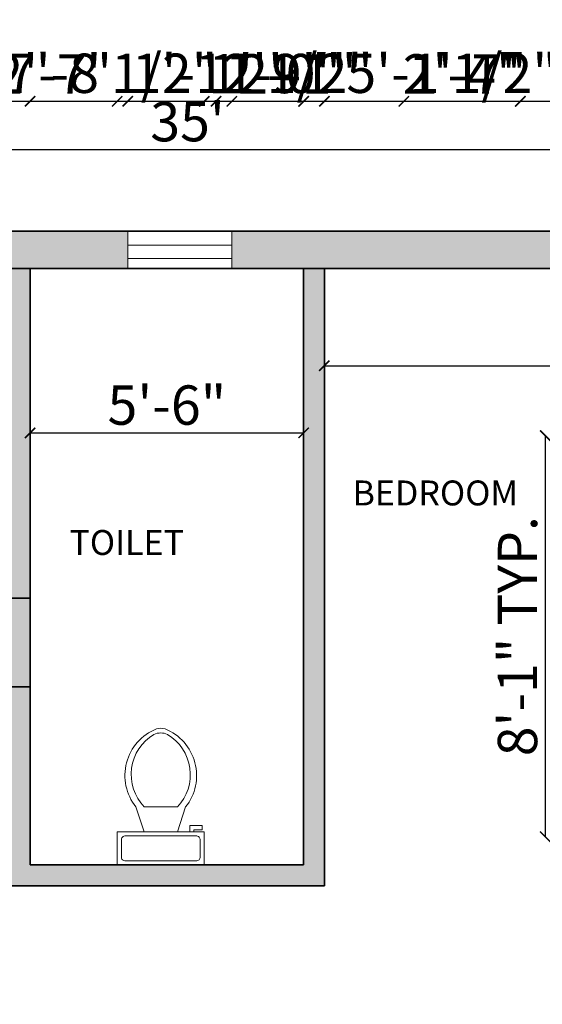
# Model space of a CAD drawing. Units: inches. Extents: x 1704 to 2334, y 1856 to 2559.
# Tile 8 of 10: x 1925 to 2051, y 2321 to 2559. Entities that reach past the tile are written whole.
import ezdxf

# ---------------------------------------------------------------- set-up
doc = ezdxf.new("R2010")
doc.units = ezdxf.units.IN
for name, color, linetype, lineweight in [('A-ANNO-DIMS', 2, 'Continuous', 18), ('A-AREA-IDEN', 7, 'Continuous', 18), ('A-FLOR-FIXT', 9, 'Continuous', 18), ('A-WALL', 7, 'Continuous', 35), ('WINDOW', 6, 'Continuous', 18)]:
    doc.layers.add(name, color=color, linetype=linetype, lineweight=lineweight)
doc.layers.add('A-WALL-PATT', color=18, linetype='Continuous', lineweight=13, true_color=0x000000)
doc.styles.get("Standard").update_dxf_attribs({"font": 'arial.ttf'})
doc.dimstyles.new('ISO-25', dxfattribs={"dimtxt": 9.5, "dimasz": 2.5, "dimexe": 1.25, "dimexo": 0.625, "dimtad": 1, "dimdec": 0, "dimlunit": 4, "dimtxsty": 'Standard', "dimblk": 'ARCHTICK', "dimcen": 2.5, "dimse1": 1, "dimse2": 1, "dimclrd": 3, "dimadec": 0, "dimazin": 0, "dimtfac": 1, "dimtdec": 0, "dimtmove": 0, "dimatfit": 3, "dimfxl": 1, "dimarcsym": 0})

# ---------------------------------------------------------------- blocks, each defined once
blk = doc.blocks.new('*U4')
for p, q in [((9.5, -6), (9.5, -2)), ((-10, -8.5), (-8, -8.5)), ((-10, -9.5), (-10, -8.5)), ((-7, -9.5), (-10, -9.5)), ((-8, -8.5), (-8, -8)), ((-7, -8), (-7, -9.5)), ((-4, -8), (-6, -14)), ((4, -8), (6, -14)), ((4, -14), (-4, -14))]:
    blk.add_line(p, q)
blk.add_lwpolyline([(10.5, -8), (10.5, 0), (-10.5, 0), (-10.5, -8)], close=True)
for points in [[(-9.5, -2), (-9.5, -6)], [(8.5, -1), (-8.5, -1)], [(-8.5, -7), (8.5, -7)]]:
    blk.add_lwpolyline(points)
for centre, radius, start, end in [((-8.62, -1.88), 0.884, 81.8699, 188.1301), ((8.62, -1.88), 0.884, 351.8699, 98.1301), ((-8.62, -6.12), 0.884, 171.8699, 278.1301), ((8.62, -6.12), 0.884, 261.8699, 8.1301), ((3.52, -21.58), 12.17, 141.4691, 247.9714), ((4.2, -21.82), 11.33, 136.3677, 238.9468), ((-3.52, -21.58), 12.17, 292.0284, 38.5307), ((-4.2, -21.82), 11.33, 301.053, 43.6321), ((0, -27.88), 4, 245.7318, 294.2682), ((0, -29), 4, 254.8605, 285.1395)]:
    blk.add_arc(centre, radius, start, end)
blk = doc.blocks.new('_ArchTick')
at = {"color": 0, "linetype": 'ByBlock', "const_width": 0.15}
blk.add_lwpolyline([(-0.5, -0.5), (0.5, 0.5)], dxfattribs=at)
blk = doc.blocks.new('*D13')
at = {"layer": 'A-ANNO-DIMS', "color": 0, "lineweight": -2, "transparency": 16777216}
blk.add_line((1927.01, 2459.35), (1993.01, 2459.35), dxfattribs=at)
at = {"layer": 'Defpoints', "color": 0, "transparency": 16777216}
for p in [(1993.01, 2459.35), (1927.01, 2452.59), (1993.01, 2452.59)]:
    blk.add_point(p, dxfattribs=at)
at = {"layer": 'A-ANNO-DIMS', "color": 0, "lineweight": -2, "transparency": 16777216, "xscale": 2.5, "yscale": 2.5, "zscale": 2.5, "rotation": 180}
blk.add_blockref('_ArchTick', (1927.01, 2459.35), dxfattribs=at)
at = {"layer": 'A-ANNO-DIMS', "color": 0, "lineweight": -2, "transparency": 16777216, "xscale": 2.5, "yscale": 2.5, "zscale": 2.5}
blk.add_blockref('_ArchTick', (1993.01, 2459.35), dxfattribs=at)
at = {"layer": 'A-ANNO-DIMS', "color": 0, "transparency": 16777216, "insert": (1960.01, 2464.83), "char_height": 9.5, "attachment_point": 5}
blk.add_mtext('5\'-6"', dxfattribs=at)
blk = doc.blocks.new('*D14')
at = {"layer": 'A-ANNO-DIMS', "color": 0, "lineweight": -2, "transparency": 16777216}
blk.add_line((1998.01, 2475.56), (2166.01, 2475.56), dxfattribs=at)
at = {"layer": 'Defpoints', "color": 0, "transparency": 16777216}
for p in [(2166.01, 2475.56), (1998.01, 2469.33), (2166.01, 2469.33)]:
    blk.add_point(p, dxfattribs=at)
at = {"layer": 'A-ANNO-DIMS', "color": 0, "lineweight": -2, "transparency": 16777216, "xscale": 2.5, "yscale": 2.5, "zscale": 2.5, "rotation": 180}
blk.add_blockref('_ArchTick', (1998.01, 2475.56), dxfattribs=at)
at = {"layer": 'A-ANNO-DIMS', "color": 0, "lineweight": -2, "transparency": 16777216, "xscale": 2.5, "yscale": 2.5, "zscale": 2.5}
blk.add_blockref('_ArchTick', (2166.01, 2475.56), dxfattribs=at)
at = {"layer": 'A-ANNO-DIMS', "color": 0, "transparency": 16777216, "insert": (2082.01, 2480.96), "char_height": 9.5, "attachment_point": 5}
blk.add_mtext("14'", dxfattribs=at)
blk = doc.blocks.new('*D22')
at = {"layer": 'A-ANNO-DIMS', "color": 0, "lineweight": -2, "transparency": 16777216}
blk.add_line((1755.01, 2527.77), (2175.01, 2527.77), dxfattribs=at)
at = {"layer": 'Defpoints', "color": 0, "transparency": 16777216}
for p in [(2175.01, 2527.77), (1755.01, 2508.04), (2175.01, 2508.04)]:
    blk.add_point(p, dxfattribs=at)
at = {"layer": 'A-ANNO-DIMS', "color": 0, "lineweight": -2, "transparency": 16777216, "xscale": 2.5, "yscale": 2.5, "zscale": 2.5, "rotation": 180}
blk.add_blockref('_ArchTick', (1755.01, 2527.77), dxfattribs=at)
at = {"layer": 'A-ANNO-DIMS', "color": 0, "lineweight": -2, "transparency": 16777216, "xscale": 2.5, "yscale": 2.5, "zscale": 2.5}
blk.add_blockref('_ArchTick', (2175.01, 2527.77), dxfattribs=at)
at = {"layer": 'A-ANNO-DIMS', "color": 0, "transparency": 16777216, "insert": (1965.01, 2533.25), "char_height": 9.5, "attachment_point": 5}
blk.add_mtext("35'", dxfattribs=at)
blk = doc.blocks.new('*D25')
at = {"layer": 'A-ANNO-DIMS', "color": 3, "lineweight": -2, "transparency": 16777216}
blk.add_line((2051.3, 2458.69), (2051.3, 2361.85), dxfattribs=at)
at = {"layer": 'Defpoints', "color": 0, "transparency": 16777216}
for p in [(2066.27, 2458.69), (2051.3, 2361.85), (2066.27, 2361.85)]:
    blk.add_point(p, dxfattribs=at)
at = {"layer": 'A-ANNO-DIMS', "color": 3, "lineweight": -2, "transparency": 16777216, "xscale": 2.5, "yscale": 2.5, "zscale": 2.5}
for p, rotation in [((2051.3, 2458.69), 90), ((2051.3, 2361.85), 270)]:
    blk.add_blockref('_ArchTick', p, dxfattribs=dict(at, rotation=rotation))
at = {"layer": 'A-ANNO-DIMS', "color": 0, "transparency": 16777216, "insert": (2045.83, 2410.27), "char_height": 9.5, "attachment_point": 5, "rotation": 90}
blk.add_mtext('8\'-1" TYP.', dxfattribs=at)
blk = doc.blocks.new('*D49')
at = {"layer": 'A-ANNO-DIMS', "color": 3, "lineweight": -2, "transparency": 16777216}
for p, q in [((1998.01, 2539.39), (2017.2, 2539.39)), ((2017.2, 2539.39), (2045.31, 2539.39))]:
    blk.add_line(p, q, dxfattribs=at)
at = {"layer": 'Defpoints', "color": 0, "transparency": 16777216}
for p in [(2017.2, 2539.39), (1998.01, 2117.04), (2017.2, 2117.04)]:
    blk.add_point(p, dxfattribs=at)
at = {"layer": 'A-ANNO-DIMS', "color": 3, "lineweight": -2, "transparency": 16777216, "xscale": 2.5, "yscale": 2.5, "zscale": 2.5, "rotation": 180}
blk.add_blockref('_ArchTick', (1998.01, 2539.39), dxfattribs=at)
at = {"layer": 'A-ANNO-DIMS', "color": 3, "lineweight": -2, "transparency": 16777216, "xscale": 2.5, "yscale": 2.5, "zscale": 2.5}
blk.add_blockref('_ArchTick', (2017.2, 2539.39), dxfattribs=at)
at = {"layer": 'A-ANNO-DIMS', "color": 0, "transparency": 16777216, "insert": (2032.51, 2544.78), "char_height": 9.5, "attachment_point": 5}
blk.add_mtext('1\'-7"', dxfattribs=at)
blk = doc.blocks.new('*D50')
at = {"layer": 'A-ANNO-DIMS', "color": 3, "lineweight": -2, "transparency": 16777216}
blk.add_line((2017.2, 2539.39), (2045.28, 2539.39), dxfattribs=at)
at = {"layer": 'Defpoints', "color": 0, "transparency": 16777216}
for p in [(2045.28, 2539.39), (2017.2, 2117.04), (2045.28, 2117.04)]:
    blk.add_point(p, dxfattribs=at)
at = {"layer": 'A-ANNO-DIMS', "color": 3, "lineweight": -2, "transparency": 16777216, "xscale": 2.5, "yscale": 2.5, "zscale": 2.5, "rotation": 180}
blk.add_blockref('_ArchTick', (2017.2, 2539.39), dxfattribs=at)
at = {"layer": 'A-ANNO-DIMS', "color": 3, "lineweight": -2, "transparency": 16777216, "xscale": 2.5, "yscale": 2.5, "zscale": 2.5}
blk.add_blockref('_ArchTick', (2045.28, 2539.39), dxfattribs=at)
at = {"layer": 'A-ANNO-DIMS', "color": 0, "transparency": 16777216, "insert": (2031.24, 2544.78), "char_height": 9.5, "attachment_point": 5}
blk.add_mtext('2\'-4"', dxfattribs=at)
blk = doc.blocks.new('*D51')
at = {"layer": 'A-ANNO-DIMS', "color": 3, "lineweight": -2, "transparency": 16777216}
for p, q in [((2045.28, 2539.39), (2054.53, 2539.39)), ((2054.53, 2539.39), (2105.67, 2539.39))]:
    blk.add_line(p, q, dxfattribs=at)
at = {"layer": 'Defpoints', "color": 0, "transparency": 16777216}
for p in [(2054.53, 2539.39), (2045.28, 2117.04), (2054.53, 2117.04)]:
    blk.add_point(p, dxfattribs=at)
at = {"layer": 'A-ANNO-DIMS', "color": 3, "lineweight": -2, "transparency": 16777216, "xscale": 2.5, "yscale": 2.5, "zscale": 2.5, "rotation": 180}
blk.add_blockref('_ArchTick', (2045.28, 2539.39), dxfattribs=at)
at = {"layer": 'A-ANNO-DIMS', "color": 3, "lineweight": -2, "transparency": 16777216, "xscale": 2.5, "yscale": 2.5, "zscale": 2.5}
blk.add_blockref('_ArchTick', (2054.53, 2539.39), dxfattribs=at)
at = {"layer": 'A-ANNO-DIMS', "color": 0, "transparency": 16777216, "insert": (2081.35, 2544.93), "char_height": 9.5, "attachment_point": 5}
blk.add_mtext('0\'-9 1/2"', dxfattribs=at)
blk = doc.blocks.new('*D55')
at = {"layer": 'A-ANNO-DIMS', "color": 3, "lineweight": -2, "transparency": 16777216}
for p, q in [((1927.01, 2539.39), (1950.56, 2539.39)), ((1950.56, 2539.39), (2008.19, 2539.39))]:
    blk.add_line(p, q, dxfattribs=at)
at = {"layer": 'Defpoints', "color": 0, "transparency": 16777216}
for p in [(1950.56, 2539.39), (1927.01, 2499.04), (1950.56, 2499.04)]:
    blk.add_point(p, dxfattribs=at)
at = {"layer": 'A-ANNO-DIMS', "color": 3, "lineweight": -2, "transparency": 16777216, "xscale": 2.5, "yscale": 2.5, "zscale": 2.5, "rotation": 180}
blk.add_blockref('_ArchTick', (1927.01, 2539.39), dxfattribs=at)
at = {"layer": 'A-ANNO-DIMS', "color": 3, "lineweight": -2, "transparency": 16777216, "xscale": 2.5, "yscale": 2.5, "zscale": 2.5}
blk.add_blockref('_ArchTick', (1950.56, 2539.39), dxfattribs=at)
at = {"layer": 'A-ANNO-DIMS', "color": 0, "transparency": 16777216, "insert": (1980.63, 2544.93), "char_height": 9.5, "attachment_point": 5}
blk.add_mtext('1\'-11 1/2"', dxfattribs=at)
blk = doc.blocks.new('*D56')
at = {"layer": 'A-ANNO-DIMS', "color": 3, "lineweight": -2, "transparency": 16777216}
for p, q in [((1950.56, 2539.39), (1975.68, 2539.39)), ((1975.68, 2539.39), (2004.85, 2539.39))]:
    blk.add_line(p, q, dxfattribs=at)
at = {"layer": 'Defpoints', "color": 0, "transparency": 16777216}
for p in [(1975.68, 2539.39), (1950.56, 2499.04), (1975.68, 2499.04)]:
    blk.add_point(p, dxfattribs=at)
at = {"layer": 'A-ANNO-DIMS', "color": 3, "lineweight": -2, "transparency": 16777216, "xscale": 2.5, "yscale": 2.5, "zscale": 2.5, "rotation": 180}
blk.add_blockref('_ArchTick', (1950.56, 2539.39), dxfattribs=at)
at = {"layer": 'A-ANNO-DIMS', "color": 3, "lineweight": -2, "transparency": 16777216, "xscale": 2.5, "yscale": 2.5, "zscale": 2.5}
blk.add_blockref('_ArchTick', (1975.68, 2539.39), dxfattribs=at)
at = {"layer": 'A-ANNO-DIMS', "color": 0, "transparency": 16777216, "insert": (1991.52, 2544.78), "char_height": 9.5, "attachment_point": 5}
blk.add_mtext('2\'-1"', dxfattribs=at)
blk = doc.blocks.new('*D57')
at = {"layer": 'A-ANNO-DIMS', "color": 3, "lineweight": -2, "transparency": 16777216}
blk.add_line((1998.01, 2539.39), (2059.64, 2539.39), dxfattribs=at)
at = {"layer": 'Defpoints', "color": 0, "transparency": 16777216}
for p in [(2059.64, 2539.39), (1998.01, 2499.04), (2059.64, 2499.04)]:
    blk.add_point(p, dxfattribs=at)
at = {"layer": 'A-ANNO-DIMS', "color": 3, "lineweight": -2, "transparency": 16777216, "xscale": 2.5, "yscale": 2.5, "zscale": 2.5, "rotation": 180}
blk.add_blockref('_ArchTick', (1998.01, 2539.39), dxfattribs=at)
at = {"layer": 'A-ANNO-DIMS', "color": 3, "lineweight": -2, "transparency": 16777216, "xscale": 2.5, "yscale": 2.5, "zscale": 2.5}
blk.add_blockref('_ArchTick', (2059.64, 2539.39), dxfattribs=at)
at = {"layer": 'A-ANNO-DIMS', "color": 0, "transparency": 16777216, "insert": (2028.82, 2544.93), "char_height": 9.5, "attachment_point": 5}
blk.add_mtext('5\'-1 1/2"', dxfattribs=at)
blk = doc.blocks.new('*D64')
at = {"layer": 'A-ANNO-DIMS', "color": 3, "lineweight": -2, "transparency": 16777216}
for p, q in [((1948.02, 2539.39), (1971.87, 2539.39)), ((1971.87, 2539.39), (2001.04, 2539.39))]:
    blk.add_line(p, q, dxfattribs=at)
at = {"layer": 'Defpoints', "color": 0, "transparency": 16777216}
for p in [(1971.87, 2539.39), (1948.02, 2153.04), (1971.87, 2153.04)]:
    blk.add_point(p, dxfattribs=at)
at = {"layer": 'A-ANNO-DIMS', "color": 3, "lineweight": -2, "transparency": 16777216, "xscale": 2.5, "yscale": 2.5, "zscale": 2.5, "rotation": 180}
blk.add_blockref('_ArchTick', (1948.02, 2539.39), dxfattribs=at)
at = {"layer": 'A-ANNO-DIMS', "color": 3, "lineweight": -2, "transparency": 16777216, "xscale": 2.5, "yscale": 2.5, "zscale": 2.5}
blk.add_blockref('_ArchTick', (1971.87, 2539.39), dxfattribs=at)
at = {"layer": 'A-ANNO-DIMS', "color": 0, "transparency": 16777216, "insert": (1987.71, 2544.86), "char_height": 9.5, "attachment_point": 5}
blk.add_mtext('2\'-0"', dxfattribs=at)
blk = doc.blocks.new('*D69')
at = {"layer": 'A-ANNO-DIMS', "color": 3, "lineweight": -2, "transparency": 16777216}
blk.add_line((2206.36, 2355.04), (2206.36, 2398.02), dxfattribs=at)
at = {"layer": 'Defpoints', "color": 0, "transparency": 16777216}
for p in [(1927.01, 2398.02), (2206.36, 2398.02), (1927.01, 2355.04)]:
    blk.add_point(p, dxfattribs=at)
at = {"layer": 'A-ANNO-DIMS', "color": 3, "lineweight": -2, "transparency": 16777216, "xscale": 2.5, "yscale": 2.5, "zscale": 2.5}
for p, rotation in [((2206.36, 2398.02), 90), ((2206.36, 2355.04), 270)]:
    blk.add_blockref('_ArchTick', p, dxfattribs=dict(at, rotation=rotation))
at = {"layer": 'A-ANNO-DIMS', "color": 0, "transparency": 16777216, "insert": (2200.88, 2376.53), "char_height": 9.5, "attachment_point": 5, "rotation": 90}
blk.add_mtext('3\'-7"', dxfattribs=at)
blk = doc.blocks.new('*D74')
at = {"layer": 'A-ANNO-DIMS', "color": 3, "lineweight": -2, "transparency": 16777216}
blk.add_line((1916.93, 2539.39), (1948.02, 2539.39), dxfattribs=at)
at = {"layer": 'Defpoints', "color": 0, "transparency": 16777216}
for p in [(1948.02, 2539.39), (1916.93, 2153.04), (1948.02, 2153.04)]:
    blk.add_point(p, dxfattribs=at)
at = {"layer": 'A-ANNO-DIMS', "color": 3, "lineweight": -2, "transparency": 16777216, "xscale": 2.5, "yscale": 2.5, "zscale": 2.5, "rotation": 180}
blk.add_blockref('_ArchTick', (1916.93, 2539.39), dxfattribs=at)
at = {"layer": 'A-ANNO-DIMS', "color": 3, "lineweight": -2, "transparency": 16777216, "xscale": 2.5, "yscale": 2.5, "zscale": 2.5}
blk.add_blockref('_ArchTick', (1948.02, 2539.39), dxfattribs=at)
at = {"layer": 'A-ANNO-DIMS', "color": 0, "transparency": 16777216, "insert": (1932.47, 2544.78), "char_height": 9.5, "attachment_point": 5}
blk.add_mtext('2\'-7"', dxfattribs=at)
blk = doc.blocks.new('*D79')
at = {"layer": 'A-ANNO-DIMS', "color": 3, "lineweight": -2, "transparency": 16777216}
blk.add_line((1723.66, 2350.04), (1723.66, 2319.04), dxfattribs=at)
at = {"layer": 'Defpoints', "color": 0, "transparency": 16777216}
for p in [(1998.01, 2350.04), (1723.66, 2319.04), (1993.01, 2319.04)]:
    blk.add_point(p, dxfattribs=at)
at = {"layer": 'A-ANNO-DIMS', "color": 3, "lineweight": -2, "transparency": 16777216, "xscale": 2.5, "yscale": 2.5, "zscale": 2.5}
for p, rotation in [((1723.66, 2350.04), 90), ((1723.66, 2319.04), 270)]:
    blk.add_blockref('_ArchTick', p, dxfattribs=dict(at, rotation=rotation))
at = {"layer": 'A-ANNO-DIMS', "color": 0, "transparency": 16777216, "insert": (1718.27, 2334.54), "char_height": 9.5, "attachment_point": 5, "rotation": 90}
blk.add_mtext('2\'-7"', dxfattribs=at)
blk = doc.blocks.new('*D80')
at = {"layer": 'A-ANNO-DIMS', "color": 3, "lineweight": -2, "transparency": 16777216}
blk.add_line((1900.32, 2539.39), (1993.01, 2539.39), dxfattribs=at)
at = {"layer": 'Defpoints', "color": 0, "transparency": 16777216}
for p in [(1993.01, 2539.39), (1900.32, 2273.04), (1993.01, 2273.04)]:
    blk.add_point(p, dxfattribs=at)
at = {"layer": 'A-ANNO-DIMS', "color": 3, "lineweight": -2, "transparency": 16777216, "xscale": 2.5, "yscale": 2.5, "zscale": 2.5, "rotation": 180}
blk.add_blockref('_ArchTick', (1900.32, 2539.39), dxfattribs=at)
at = {"layer": 'A-ANNO-DIMS', "color": 3, "lineweight": -2, "transparency": 16777216, "xscale": 2.5, "yscale": 2.5, "zscale": 2.5}
blk.add_blockref('_ArchTick', (1993.01, 2539.39), dxfattribs=at)
at = {"layer": 'A-ANNO-DIMS', "color": 0, "transparency": 16777216, "insert": (1946.66, 2544.93), "char_height": 9.5, "attachment_point": 5}
blk.add_mtext('7\'-8 1/2"', dxfattribs=at)
blk = doc.blocks.new('*D84')
at = {"layer": 'A-ANNO-DIMS', "color": 3, "lineweight": -2, "transparency": 16777216}
blk.add_line((2206.36, 2388.04), (2206.36, 2355.04), dxfattribs=at)
at = {"layer": 'Defpoints', "color": 0, "transparency": 16777216}
for p in [(1958.54, 2388.04), (1969.04, 2355.04), (2206.36, 2355.04)]:
    blk.add_point(p, dxfattribs=at)
at = {"layer": 'A-ANNO-DIMS', "color": 3, "lineweight": -2, "transparency": 16777216, "xscale": 2.5, "yscale": 2.5, "zscale": 2.5}
for p, rotation in [((2206.36, 2388.04), 90), ((2206.36, 2355.04), 270)]:
    blk.add_blockref('_ArchTick', p, dxfattribs=dict(at, rotation=rotation))
at = {"layer": 'A-ANNO-DIMS', "color": 0, "transparency": 16777216, "insert": (2200.88, 2371.54), "char_height": 9.5, "attachment_point": 5, "rotation": 90}
blk.add_mtext('2\'-9"', dxfattribs=at)
blk = doc.blocks.new('*D85')
at = {"layer": 'A-ANNO-DIMS', "color": 3, "lineweight": -2, "transparency": 16777216}
for p, q in [((1948.04, 2539.39), (1969.04, 2539.39)), ((1969.04, 2539.39), (1997.15, 2539.39))]:
    blk.add_line(p, q, dxfattribs=at)
at = {"layer": 'Defpoints', "color": 0, "transparency": 16777216}
for p in [(1969.04, 2539.39), (1948.04, 2363.04), (1969.04, 2363.04)]:
    blk.add_point(p, dxfattribs=at)
at = {"layer": 'A-ANNO-DIMS', "color": 3, "lineweight": -2, "transparency": 16777216, "xscale": 2.5, "yscale": 2.5, "zscale": 2.5, "rotation": 180}
blk.add_blockref('_ArchTick', (1948.04, 2539.39), dxfattribs=at)
at = {"layer": 'A-ANNO-DIMS', "color": 3, "lineweight": -2, "transparency": 16777216, "xscale": 2.5, "yscale": 2.5, "zscale": 2.5}
blk.add_blockref('_ArchTick', (1969.04, 2539.39), dxfattribs=at)
at = {"layer": 'A-ANNO-DIMS', "color": 0, "transparency": 16777216, "insert": (1984.35, 2544.86), "char_height": 9.5, "attachment_point": 5}
blk.add_mtext('1\'-9"', dxfattribs=at)

msp = doc.modelspace()

# ---------------------------------------------------------------- hatches: boundary and pattern name
at = {"layer": 'A-WALL-PATT'}
h = msp.add_hatch(color=256, dxfattribs=at)
h.dxf.hatch_style = 1
h.paths.add_polyline_path([(1764.01, 2204.96), (1755.01, 2204.96), (1755.01, 2115.31), (1764.01, 2115.31)])
h.paths.add_polyline_path([(1764.01, 2076.84), (1755.01, 2076.84), (1755.01, 1968.04), (1794.77, 1968.04), (1794.77, 1977.04), (1764.01, 1977.04)])
h.paths.add_polyline_path([(1927.01, 1977.04), (1927.01, 2069.24), (1993.01, 2069.24), (1993.01, 1977.04)], flags=16)
h.paths.add_polyline_path([(1927.01, 2074.24), (1927.01, 2148.04), (1993.01, 2148.04), (1993.01, 2074.24)], flags=16)
h.paths.add_polyline_path([(1764.01, 2318.65), (1755.01, 2318.65), (1755.01, 2247.44), (1764.01, 2247.44)])
h.paths.add_polyline_path([(1764.01, 2499.04), (1798.75, 2499.04), (1798.75, 2508.04), (1755.01, 2508.04), (1755.01, 2336.43), (1764.01, 2336.43)])
h.paths.add_polyline_path([(1950.56, 2508.04), (1847.17, 2508.04), (1847.17, 2499.04), (1950.56, 2499.04)])
h.paths.add_polyline_path([(2059.64, 2508.04), (1975.68, 2508.04), (1975.68, 2499.04), (2059.64, 2499.04)])
h.paths.add_polyline_path([(2175.01, 2508.04), (2108.25, 2508.04), (2108.25, 2499.04), (2166.01, 2499.04), (2166.01, 1977.04), (2166.01, 1972.26), (2166.01, 1968.04), (2175.01, 1968.04)])
h.paths.add_polyline_path([(2166.01, 2319.04), (1993.01, 2319.04), (1993.01, 2273.04), (1998.01, 2273.04), (1998.01, 2314.04), (2166.01, 2314.04)])
h.paths.add_polyline_path([(2054.53, 2117.04), (1998.01, 2117.04), (1998.01, 2112.04), (2054.53, 2112.04)])
h.paths.add_polyline_path([(2166.01, 2117.04), (2105.53, 2117.04), (2105.53, 2112.04), (2166.01, 2112.04)])
h.paths.add_polyline_path([(1927.01, 2499.04), (1922.01, 2499.04), (1922.01, 2355.04), (1764.01, 2355.04), (1764.01, 2350.04), (1804.01, 2350.04), (1804.01, 2278.04), (1764.01, 2278.04), (1764.01, 2273.04), (1870.51, 2273.04), (1870.51, 2278.04), (1870.51, 2350.04), (1865.51, 2350.04), (1865.51, 2278.04), (1809.01, 2278.04), (1809.01, 2350.04), (1922.01, 2350.04), (1927.01, 2350.04), (1998.01, 2350.04), (1998.01, 2499.04), (1993.01, 2499.04), (1993.01, 2355.04), (1927.01, 2355.04)])
h.paths.add_polyline_path([(2131.1, 2203.36), (2144.85, 2203.36), (2144.85, 2212.38), (2131.1, 2212.38)], flags=25)
h.paths.add_polyline_path([(2010.94, 2265.21), (2036.85, 2265.21), (2036.85, 2274.23), (2010.94, 2274.23)], flags=9)
h.paths.add_polyline_path([(2010.9, 2274.71), (2056.95, 2274.71), (2056.95, 2284.04), (2010.9, 2284.04)], flags=25)
h.paths.add_polyline_path([(2003.27, 2440.18), (2049.79, 2440.18), (2049.79, 2449.51), (2003.27, 2449.51)], flags=9)
h.paths.add_polyline_path([(1934.96, 2428.22), (1967.48, 2428.22), (1967.48, 2437.55), (1934.96, 2437.55)], flags=25)
h.paths.add_polyline_path([(1778.93, 2466.23), (1827.79, 2466.23), (1827.79, 2475.56), (1778.93, 2475.56)], flags=25)
h.paths.add_polyline_path([(1938.32, 2043.05), (1970.37, 2043.05), (1970.37, 2052.39), (1938.32, 2052.39)], flags=8)
h.paths.add_polyline_path([(1932.21, 2095.38), (1956.75, 2095.38), (1956.75, 2104.56), (1932.21, 2104.56)], flags=8)
h.paths.add_polyline_path([(1888.97, 2148.04), (1888.97, 2153.04), (1764.01, 2153.04), (1764.01, 2148.04)])
h.paths.add_polyline_path([(1922.01, 2059.61), (1927.01, 2059.61), (1927.01, 2044.47), (1922.01, 2044.47), (1922.01, 1977.04), (1857.04, 1977.04), (1857.04, 1968.04), (1998.01, 1968.04), (1998.01, 1977.04), (1998.01, 2153.04), (1916.93, 2153.04), (1916.93, 2148.04), (1922.01, 2148.04)])

# ---------------------------------------------------------------- linework, layer by layer
at = {"layer": 'A-WALL'}
for p, q in [((1764.01, 2499.04), (2166.01, 2499.04)), ((1927.01, 2355.04), (1927.01, 2499.04)), ((1993.01, 2499.04), (1993.01, 2355.04)), ((1993.01, 2355.04), (1993.01, 2499.04)), ((1998.01, 2499.04), (1998.01, 2350.04)), ((1998.01, 2350.04), (1998.01, 2499.04)), ((1927.01, 2419.48), (1922.01, 2419.48)), ((1927.01, 2398.02), (1922.01, 2398.02)), ((1927.01, 2355.04), (1993.01, 2355.04)), ((1927.01, 2350.04), (1922.01, 2350.04)), ((1927.01, 2350.04), (1998.01, 2350.04))]:
    msp.add_line(p, q, dxfattribs=at)
msp.add_lwpolyline([(1998.01, 1968.04), (1755.01, 1968.04), (1755.01, 2508.04), (2175.01, 2508.04), (2175.01, 1968.04), (2166.01, 1968.04)], dxfattribs=at)
at = {"layer": 'WINDOW'}
for p, q in [((1950.56, 2508.04), (1950.56, 2499.04)), ((1975.68, 2508.04), (1950.56, 2508.04)), ((1975.68, 2499.04), (1975.68, 2508.04)), ((1975.68, 2504.66), (1950.56, 2504.66)), ((1975.68, 2501.48), (1950.56, 2501.48)), ((1950.56, 2499.04), (1975.68, 2499.04))]:
    msp.add_line(p, q, dxfattribs=at)

# ---------------------------------------------------------------- block references
at = {"layer": 'A-FLOR-FIXT', "rotation": 180}
msp.add_blockref('*U4', (1958.54, 2355.04), dxfattribs=at)

# ---------------------------------------------------------------- texts
at = {"layer": 'A-AREA-IDEN'}
for s, p in [('BEDROOM', (2004.82, 2441.84)), ('TOILET', (1936.52, 2429.88))]:
    msp.add_text(s, height=6.013, dxfattribs=at).set_placement(p)

# ---------------------------------------------------------------- dimensions: what is measured, and where the dimension line sits
at = {"layer": 'A-ANNO-DIMS'}
for base, p1, p2, override, picture, middle in [((1993.01, 2539.39), (1900.32, 2273.04), (1993.01, 2273.04), {"dimdec": 1, "dimlfac": 1, "dimrnd": 0, "dimzin": 1, "dimdsep": 46, "dimlunit": 4, "dimfrac": 2}, '*D80', (1946.66, 2544.93)), ((1950.5636, 2539.3895), (1927.0097, 2499.0395), (1950.5636, 2499.0395), {"dimdec": 1, "dimlfac": 1, "dimrnd": 0, "dimzin": 1, "dimdsep": 46, "dimlunit": 4, "dimfrac": 2}, '*D55', (1980.6269, 2544.9265)), ((2059.64, 2539.39), (1998.01, 2499.04), (2059.64, 2499.04), {"dimdec": 1, "dimlfac": 1, "dimrnd": 0, "dimzin": 1, "dimdsep": 46, "dimlunit": 4, "dimfrac": 2}, '*D57', (2028.82, 2544.93)), ((2054.5307, 2539.3895), (2045.2758, 2117.0395), (2054.5307, 2117.0395), {"dimdec": 1, "dimlfac": 1, "dimrnd": 0, "dimzin": 1, "dimdsep": 46, "dimlunit": 4, "dimfrac": 2}, '*D51', (2081.3506, 2544.9265)), ((1948.02, 2539.39), (1916.93, 2153.04), (1948.02, 2153.04), {"dimdec": 1, "dimlfac": 1, "dimrnd": 0, "dimzin": 1, "dimdsep": 46, "dimlunit": 4, "dimfrac": 2}, '*D74', (1932.47, 2544.78)), ((1971.8732, 2539.3895), (1948.0187, 2153.0395), (1971.8732, 2153.0395), {"dimdec": 1, "dimlfac": 1, "dimrnd": 0, "dimzin": 1, "dimdsep": 46, "dimlunit": 4, "dimfrac": 2}, '*D64', (1987.7059, 2544.8649)), ((1969.04, 2539.39), (1948.04, 2363.04), (1969.04, 2363.04), {"dimdec": 1, "dimlfac": 1, "dimrnd": 0, "dimzin": 1, "dimdsep": 46, "dimlunit": 4, "dimfrac": 2}, '*D85', (1984.35, 2544.86)), ((1975.68, 2539.39), (1950.56, 2499.04), (1975.68, 2499.04), {"dimdec": 1, "dimlfac": 1, "dimrnd": 0, "dimzin": 1, "dimdsep": 46, "dimlunit": 4, "dimfrac": 2}, '*D56', (1991.52, 2544.78)), ((2017.2, 2539.39), (1998.01, 2117.04), (2017.2, 2117.04), {"dimdec": 1, "dimlfac": 1, "dimrnd": 0, "dimzin": 1, "dimdsep": 46, "dimlunit": 4, "dimfrac": 2}, '*D49', (2032.51, 2544.78)), ((2045.28, 2539.39), (2017.2, 2117.04), (2045.28, 2117.04), {"dimdec": 1, "dimlfac": 1, "dimrnd": 0, "dimzin": 1, "dimdsep": 46, "dimlunit": 4, "dimfrac": 2}, '*D50', (2031.24, 2544.78)), ((2175.01, 2527.77), (1755.01, 2508.04), (2175.01, 2508.04), {"dimclrd": 0, "dimclre": 0, "dimclrt": 0}, '*D22', (1965.01, 2533.25)), ((2166.01, 2475.56), (1998.01, 2469.33), (2166.01, 2469.33), {"dimclrd": 0, "dimclre": 0, "dimclrt": 0}, '*D14', (2082.01, 2480.96)), ((1993.01, 2459.35), (1927.01, 2452.59), (1993.01, 2452.59), {"dimclrd": 0, "dimclre": 0, "dimclrt": 0}, '*D13', (1960.01, 2464.83))]:
    dim = msp.add_linear_dim(base=base, p1=p1, p2=p2, dimstyle='ISO-25', override=override, dxfattribs=at)
    dim.commit()
    dim.dimension.update_dxf_attribs({"geometry": picture, "text_midpoint": middle})
dim = msp.add_linear_dim(base=(2051.3, 2361.85), p1=(2066.27, 2458.69), p2=(2066.27, 2361.85), angle=270, text='<> TYP.', dimstyle='ISO-25', override={"dimdec": 1, "dimlfac": 1, "dimrnd": 0, "dimzin": 1, "dimdsep": 46, "dimlunit": 4, "dimfrac": 2}, dxfattribs=at)
dim.commit()
dim.dimension.update_dxf_attribs({"geometry": '*D25', "text_midpoint": (2045.83, 2410.27)})
for base, p1, p2, picture, middle in [((2206.36, 2398.02), (1927.01, 2355.04), (1927.01, 2398.02), '*D69', (2200.88, 2376.53)), ((2206.36, 2355.04), (1958.54, 2388.04), (1969.04, 2355.04), '*D84', (2200.88, 2371.54)), ((1723.66, 2319.04), (1998.01, 2350.04), (1993.01, 2319.04), '*D79', (1718.27, 2334.54))]:
    dim = msp.add_linear_dim(base=base, p1=p1, p2=p2, angle=90, dimstyle='ISO-25', override={"dimdec": 1, "dimlfac": 1, "dimrnd": 0, "dimzin": 1, "dimdsep": 46, "dimlunit": 4, "dimfrac": 2}, dxfattribs=at)
    dim.commit()
    dim.dimension.update_dxf_attribs({"geometry": picture, "text_midpoint": middle})

doc.saveas('drawing.dxf')
